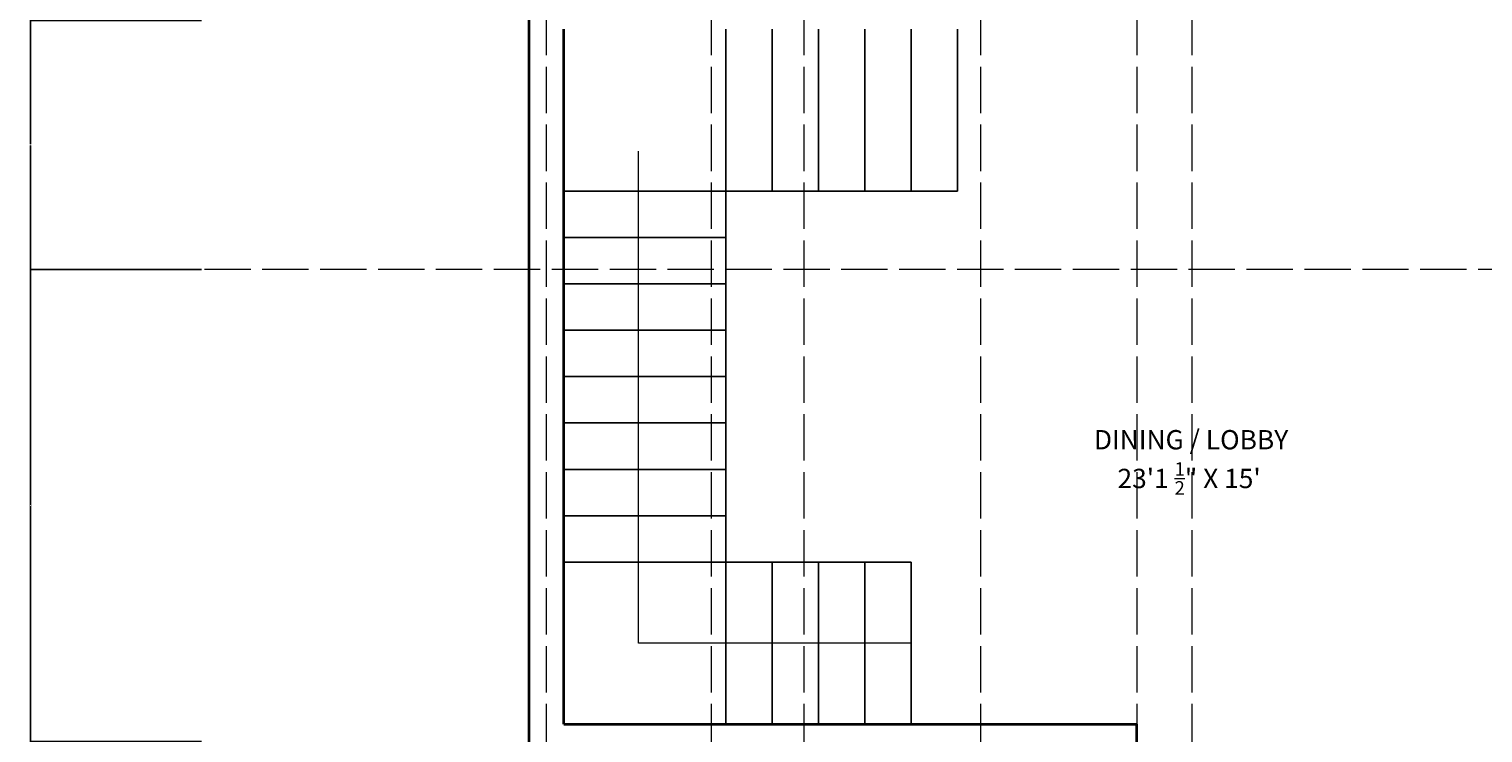
# Model space of a CAD drawing. Units: inches. Extents: x 1159 to 4240, y 1112 to 2085.
# Tile 4 of 13: x 1159 to 1535, y 1551 to 1734. Entities that reach past the tile are written whole.
import ezdxf

# ---------------------------------------------------------------- set-up
doc = ezdxf.new("R2010")
doc.units = ezdxf.units.IN
doc.linetypes.add('ACAD_ISO02W100', pattern=[15, 12, -3])
for name, color, linetype, lineweight in [('A-ANNO-DIMS', 2, 'Continuous', 18), ('A-ANNO-SYMB', 150, 'Continuous', 18), ('A-AREA-IDEN', 30, 'Continuous', 18), ('A-GRID', 8, 'ACAD_ISO02W100', 13), ('STAIRCASE', 150, 'Continuous', 25), ('WALL', 7, 'Continuous', 35)]:
    doc.layers.add(name, color=color, linetype=linetype, lineweight=lineweight)
doc.styles.get("Standard").update_dxf_attribs({"font": 'arial.ttf'})
doc.dimstyles.get("Standard").update_dxf_attribs({"dimtxt": 0.18, "dimasz": 0.18, "dimexe": 0.18, "dimexo": 0.0625, "dimgap": 0.09, "dimtad": 0, "dimtih": 1, "dimtoh": 1, "dimdec": 4, "dimzin": 0, "dimdsep": 46, "dimtxsty": 'Standard', "dimcen": 0.09, "dimadec": 0, "dimazin": 0, "dimtfac": 1, "dimtdec": 4, "dimtofl": 0, "dimtmove": 0, "dimatfit": 3, "dimfxl": 1, "dimtolj": 1, "dimtzin": 0, "dimarcsym": 0})

# ---------------------------------------------------------------- blocks, each defined once
blk = doc.blocks.new('HOUSE-35x60-WALL-LAYOUT')
for p, q in [((0, 0), (0, 720)), ((9, 306), (9, 486)), ((9, 306), (157.5, 306)), ((157.5, 190.5), (157.5, 306))]:
    blk.add_line(p, q)
blk = doc.blocks.new('STAIR-THREE-FLIGHT')
for p, q in [((42, 138), (42, 180)), ((54, 138), (54, 180)), ((66, 138), (66, 180)), ((78, 138), (78, 180)), ((90, 138), (90, 180)), ((102, 138), (102, 180)), ((0, 138), (42, 138)), ((102, 138), (42, 138)), ((42, 138), (42, 42)), ((0, 126), (42, 126)), ((0, 114), (42, 114)), ((0, 102), (42, 102)), ((0, 90), (42, 90)), ((0, 78), (42, 78)), ((0, 66), (42, 66)), ((0, 54), (42, 54)), ((0, 42), (42, 42)), ((42, 0), (42, 42)), ((42, 42), (90, 42)), ((54, 0), (54, 42)), ((66, 0), (66, 42)), ((78, 0), (78, 42)), ((90, 0), (90, 42))]:
    blk.add_line(p, q)
blk = doc.blocks.new('STAIR-PATH-ARROW')
blk.add_lwpolyline([(0, 127.38, 0, 0, 0), (0, 143.35, 0, 0, 0), (58.69, 143.35, 4, 0, 0), (70.69, 143.35, 0, 0, 0)], format="xyseb")
blk.add_lwpolyline([(70.69, 0), (0, 0), (0, 127.38)])
blk = doc.blocks.new('HOUSE-35x60-SETTING-OUT-GRID')
for p, q in [((89.32, 0), (89.32, 883.25)), ((132.07, 0), (132.07, 883.25)), ((156.07, 0), (156.07, 883.25)), ((201.82, 0), (201.82, 883.25)), ((242.32, 0), (242.32, 883.25)), ((256.57, 0), (256.57, 883.25)), ((582.7, 514.5), (0, 514.5))]:
    blk.add_line(p, q)
blk = doc.blocks.new('*D41')
at = {"layer": 'A-ANNO-DIMS', "color": 0, "lineweight": -2, "transparency": 16777216}
for p, q in [((1203.25, 1671.45), (1158.78, 1671.45)), ((1158.96, 1671.27), (1158.96, 1610.51)), ((1158.96, 1549.38), (1158.96, 1610.15)), ((1203.25, 1549.2), (1158.78, 1549.2))]:
    blk.add_line(p, q, dxfattribs=at)
at = {"layer": 'A-ANNO-DIMS', "color": 0, "lineweight": 100, "transparency": 16777216}
for points in [[(1158.93, 1671.27), (1158.99, 1671.27), (1158.96, 1671.45)], [(1158.93, 1549.38), (1158.99, 1549.38), (1158.96, 1549.2)]]:
    blk.add_solid(points, dxfattribs=at)
at = {"layer": 'Defpoints', "color": 0, "lineweight": 100, "transparency": 16777216}
for p in [(1158.96, 1671.45), (1203.31, 1671.45), (1203.31, 1549.2)]:
    blk.add_point(p, dxfattribs=at)
at = {"layer": 'A-ANNO-DIMS', "color": 0, "transparency": 16777216, "insert": (1158.96, 1610.33), "char_height": 0.18, "attachment_point": 5}
blk.add_mtext('\\A1;122.25', dxfattribs=at)
blk = doc.blocks.new('*D42')
at = {"layer": 'A-ANNO-DIMS', "color": 0, "lineweight": -2, "transparency": 16777216}
for p, q in [((1203.25, 1735.95), (1158.78, 1735.95)), ((1158.96, 1735.77), (1158.96, 1703.88)), ((1158.96, 1671.63), (1158.96, 1703.52)), ((1203.25, 1671.45), (1158.78, 1671.45))]:
    blk.add_line(p, q, dxfattribs=at)
at = {"layer": 'A-ANNO-DIMS', "color": 0, "lineweight": 100, "transparency": 16777216}
for points in [[(1158.93, 1735.77), (1158.99, 1735.77), (1158.96, 1735.95)], [(1158.93, 1671.63), (1158.99, 1671.63), (1158.96, 1671.45)]]:
    blk.add_solid(points, dxfattribs=at)
at = {"layer": 'Defpoints', "color": 0, "lineweight": 100, "transparency": 16777216}
for p in [(1158.96, 1735.95), (1203.31, 1735.95), (1203.31, 1671.45)]:
    blk.add_point(p, dxfattribs=at)
at = {"layer": 'A-ANNO-DIMS', "color": 0, "transparency": 16777216, "insert": (1158.96, 1703.7), "char_height": 0.18, "attachment_point": 5}
blk.add_mtext('\\A1;64.5', dxfattribs=at)

msp = doc.modelspace()

# ---------------------------------------------------------------- block references
at = {"layer": 'A-ANNO-SYMB'}
msp.add_blockref('STAIR-PATH-ARROW', (1316.437, 1574.702), dxfattribs=at)
at = {"layer": 'A-GRID'}
msp.add_blockref('HOUSE-35x60-SETTING-OUT-GRID', (1203.31, 1156.954), dxfattribs=at)
at = {"layer": 'STAIRCASE'}
msp.add_blockref('STAIR-THREE-FLIGHT', (1297.126, 1553.702), dxfattribs=at)
at = {"layer": 'WALL'}
msp.add_blockref('HOUSE-35x60-WALL-LAYOUT', (1288.126, 1247.702), dxfattribs=at)

# ---------------------------------------------------------------- texts
at = {"layer": 'A-AREA-IDEN', "insert": (1434.47, 1629.873), "char_height": 5, "attachment_point": 1}
msp.add_mtext_dynamic_manual_height_columns('\\A1;DINING / LOBBY\\P    23\'1 {\\H0.7x;\\S1/2;}" X 15\'', width=140.18614, gutter_width=12.5, heights=[0], dxfattribs=at)

# ---------------------------------------------------------------- dimensions: what is measured, and where the dimension line sits
at = {"layer": 'A-ANNO-DIMS'}
for base, p1, p2, override, picture, middle in [((1158.96, 1735.952), (1203.31, 1671.452), (1203.31, 1735.952), {"dimdec": 1, "dimlfac": 1, "dimrnd": 0, "dimzin": 0, "dimdsep": 46, "dimlunit": 2}, '*D42', (1158.96, 1703.702)), ((1158.96, 1671.452), (1203.31, 1549.202), (1203.31, 1671.452), {"dimdec": 2, "dimlfac": 1, "dimrnd": 0, "dimzin": 0, "dimdsep": 46, "dimlunit": 2}, '*D41', (1158.96, 1610.327))]:
    dim = msp.add_linear_dim(base=base, p1=p1, p2=p2, angle=90, dimstyle='Standard', override=override, dxfattribs=at)
    dim.commit()
    dim.dimension.update_dxf_attribs({"geometry": picture, "text_midpoint": middle})

doc.saveas('drawing.dxf')
